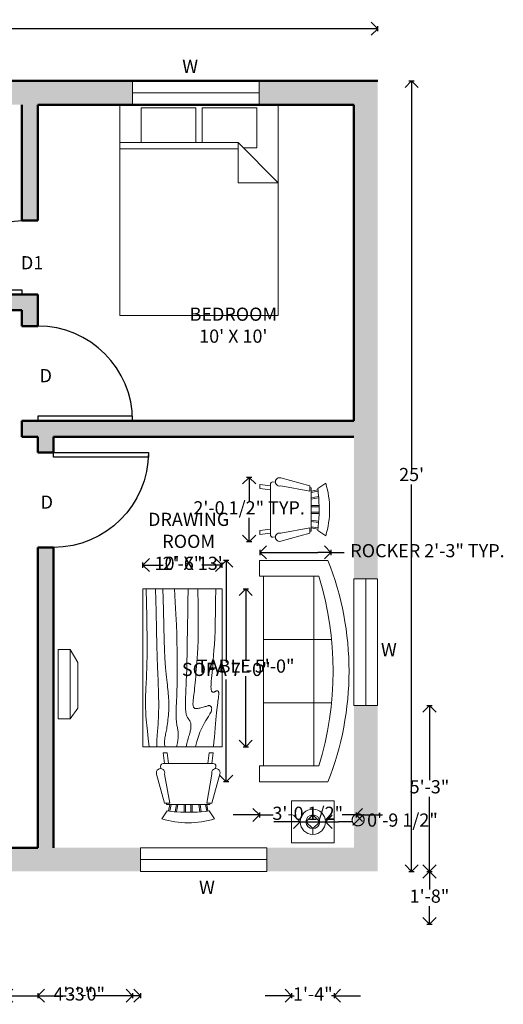
# Model space of a CAD drawing. Units: inches. Extents: x 2691 to 3149, y 584 to 962.
# Tile 3 of 3: x 2966 to 3149, y 588 to 962. Entities that reach past the tile are written whole.
import ezdxf

# ---------------------------------------------------------------- set-up
doc = ezdxf.new("R2010")
doc.units = ezdxf.units.IN
for name, color, linetype, lineweight in [('A-ANNO-DIMS', 2, 'Continuous', 18), ('A-ANNO-TEXT', 159, 'Continuous', 18), ('A-AREA-IDEN', 7, 'Continuous', 25), ('A-DOOR', 4, 'Continuous', 25), ('A-EQPM', 8, 'Continuous', 18), ('A-FURN', 8, 'Continuous', 18), ('A-GLAZ', 40, 'Continuous', 18), ('A-WALL', 254, 'Continuous', 50), ('A-WALL-PATT', 252, 'Continuous', 13)]:
    doc.layers.add(name, color=color, linetype=linetype, lineweight=lineweight)
doc.styles.get("Standard").update_dxf_attribs({"font": 'arial.ttf'})
doc.dimstyles.new('ISO-25', dxfattribs={"dimtxt": 5, "dimasz": 5, "dimexe": 1, "dimexo": 1, "dimtad": 0, "dimtih": 1, "dimtoh": 1, "dimdec": 1, "dimlunit": 3, "dimtxsty": 'Standard', "dimblk": 'OPEN90', "dimcen": 2.5, "dimclrd": 1, "dimclre": 1, "dimclrt": 1, "dimadec": 0, "dimazin": 0, "dimtfac": 1, "dimtdec": 1, "dimtmove": 0, "dimatfit": 3, "dimfxl": 1, "dimfxlon": 1, "dimarcsym": 0})

# ---------------------------------------------------------------- blocks, each defined once
blk = doc.blocks.new('*U5')
for p, q in [((0, 0), (0, -6)), ((-36, 0), (-36, -6))]:
    blk.add_line(p, q)
blk.add_lwpolyline([(0, 0), (0, 36), (-1.75, 36), (-1.75, 0)], close=True)
blk.add_arc((0, 0), 36, 90, 180)
blk = doc.blocks.new('*U4')
for p, q in [((-28, 0), (-28, -6)), ((0, 0), (0, -6))]:
    blk.add_line(p, q)
blk.add_lwpolyline([(0, 0), (0, 28), (-1.75, 28), (-1.75, 0)], close=True)
blk.add_arc((0, 0), 28, 90, 180)
blk = doc.blocks.new('Bed - Queen')
for p, q in [((0, -80.00003), (0, 0)), ((0, 0), (59.99999, 0)), ((59.99999, 0), (59.99999, -80.00003)), ((7.99999, -1.2), (28.79998, -1.2)), ((7.99999, -14.4), (7.99999, -1.2)), ((28.79998, -1.2), (28.79998, -14.4)), ((31.19999, -1.2), (51.99999, -1.2)), ((31.19999, -14.4), (31.19999, -1.2)), ((51.99999, -1.2), (51.99999, -16.4)), ((0, -14.4), (44.8, -14.4)), ((59.99999, -29.6), (44.8, -14.4)), ((44.8, -14.4), (44.8, -29.6)), ((44.8, -16.8), (0, -16.8)), ((51.99999, -16.4), (46.79936, -16.4)), ((44.8, -29.6), (59.99999, -29.6)), ((59.99999, -80.00003), (0, -80.00003))]:
    blk.add_line(p, q)
blk = doc.blocks.new('Sofa - Roundback 7 ft.')
for p, q in [((-12.00002, -32.4421), (-12.00003, -6.5971)), ((11.99997, -32.4421), (11.99998, -6.5971)), ((-36.000027, -34), (-36.000027, -11.4696)), ((-35.999844, -13.3819), (35.9998, -13.3819)), ((35.99998, -34), (35.99998, -11.4696)), ((-36.000027, -32.4421), (35.99998, -32.4421))]:
    blk.add_line(p, q)
for points in [[(-36.000027, -34), (-42.000027, -34), (-42.000027, -8)], [(41.99998, -8), (41.99998, -34), (35.99998, -34)]]:
    blk.add_lwpolyline(points)
for centre, radius, start, end in [((0, -114.25), 114.25, 68.43141, 111.5686), ((-0.00001, -127.1968), 121.1968, 72.72033, 107.2797)]:
    blk.add_arc(centre, radius, start, end)
blk = doc.blocks.new('Table - Rectangular Woodgrain 60 x 30 in.')
for p, q in [((0, 0), (0, -30)), ((60, 0), (0, 0)), ((60, -30), (60, 0)), ((0, -30), (60, -30))]:
    blk.add_line(p, q)
for points in [[(0, -2.4), (4.8155, -2.418), (9.0302, -2.4688), (12.709, -2.5477), (15.9167, -2.65), (18.7181, -2.7711), (21.1781, -2.9063), (23.3616, -3.0508), (25.3333, -3.2), (27.1477, -3.3495), (28.8172, -3.4958), (30.3437, -3.636), (31.7291, -3.7667), (32.9756, -3.8849), (34.0849, -3.9875), (35.059, -4.0714), (35.9, -4.1334), (36.6114, -4.1711), (37.2041, -4.1854), (37.6906, -4.1779), (38.0833, -4.15), (38.3948, -4.1034), (38.6375, -4.0396), (38.8239, -3.9602), (38.9666, -3.8667), (39.0764, -3.7608), (39.1573, -3.6448), (39.2116, -3.521), (39.2416, -3.3917), (39.2498, -3.2593), (39.2385, -3.1261), (39.21, -2.9944), (39.1666, -2.8667), (39.111, -2.7447), (39.0468, -2.6281), (38.978, -2.5163), (38.9083, -2.4083), (38.8418, -2.3035), (38.7823, -2.201), (38.7337, -2.1001), (38.7, -2), (38.6844, -1.9003), (38.6875, -1.8021), (38.7094, -1.707), (38.75, -1.6167), (38.8094, -1.5326), (38.8875, -1.4563), (38.9844, -1.3893), (39.1, -1.3333), (39.2351, -1.2896), (39.3937, -1.2583), (39.5804, -1.2396), (39.8, -1.2333), (40.057, -1.2396), (40.3562, -1.2583), (40.7023, -1.2896), (41.1, -1.3333), (41.5547, -1.3895), (42.0755, -1.4573), (42.6721, -1.5361), (43.3542, -1.625), (44.1316, -1.7233), (45.014, -1.8302), (46.0114, -1.9449), (47.1333, -2.0667), (48.3862, -2.1947), (49.7625, -2.3281), (51.2513, -2.4663), (52.8416, -2.6083), (54.5226, -2.7535), (56.2833, -2.9011), (58.1127, -3.0501), (60, -3.2)], [(0, -9.2), (6.5759, -9.0858), (11.9385, -9.0365), (16.2527, -9.0418), (19.6833, -9.0917), (22.3952, -9.1759), (24.5531, -9.2844), (26.322, -9.4069), (27.8666, -9.5333), (29.3241, -9.6553), (30.7203, -9.7719), (32.0532, -9.8837), (33.3208, -9.9917), (34.5213, -10.0965), (35.6526, -10.199), (36.7128, -10.2999), (37.7, -10.4), (38.6129, -10.4996), (39.4531, -10.5969), (40.223, -10.6895), (40.925, -10.775), (41.5613, -10.8512), (42.1344, -10.9156), (42.6465, -10.966), (43.1, -11), (43.4976, -11.0158), (43.8437, -11.0136), (44.143, -10.9942), (44.4, -10.9583), (44.6195, -10.9069), (44.8062, -10.8406), (44.9648, -10.7603), (45.1, -10.6667), (45.2155, -10.5598), (45.3114, -10.4365), (45.3871, -10.2929), (45.4416, -10.125), (45.4743, -9.929), (45.4844, -9.7011), (45.4709, -9.4371), (45.4333, -9.1333), (45.3716, -8.7883), (45.2896, -8.4104), (45.1919, -8.0107), (45.0833, -7.6), (44.9685, -7.1893), (44.8521, -6.7896), (44.7388, -6.4117), (44.6333, -6.0667), (44.54, -5.7628), (44.4614, -5.4979), (44.4001, -5.2675), (44.3583, -5.0667), (44.3384, -4.8909), (44.3427, -4.7354), (44.3736, -4.5956), (44.4333, -4.4667), (44.5236, -4.3453), (44.6427, -4.2333), (44.7884, -4.1339), (44.9583, -4.05), (45.1501, -3.9849), (45.3614, -3.9417), (45.59, -3.9234), (45.8333, -3.9333), (46.0915, -3.9749), (46.3734, -4.0531), (46.6906, -4.1736), (47.0542, -4.3417), (47.4756, -4.5629), (47.9661, -4.8427), (48.5372, -5.1866), (49.2, -5.6), (49.9676, -6.0844), (50.8594, -6.625), (51.8965, -7.2031), (53.1, -7.8), (54.491, -8.3969), (56.0906, -8.975), (57.9199, -9.5156), (60, -10)], [(0, -12.8), (5.1847, -12.9322), (9.6213, -13.0323), (13.3963, -13.1059), (16.5958, -13.1583), (19.3063, -13.1952), (21.614, -13.2219), (23.6054, -13.2439), (25.3666, -13.2667), (26.9728, -13.2947), (28.4531, -13.3281), (29.8256, -13.3663), (31.1083, -13.4083), (32.3191, -13.4535), (33.476, -13.501), (34.597, -13.5501), (35.7, -13.6), (36.7984, -13.6497), (37.8875, -13.6979), (38.9578, -13.743), (40, -13.7833), (41.0047, -13.8174), (41.9625, -13.8438), (42.864, -13.8607), (43.7, -13.8667), (44.4631, -13.8604), (45.1552, -13.8417), (45.7801, -13.8104), (46.3416, -13.7667), (46.8439, -13.7104), (47.2906, -13.6417), (47.6858, -13.5604), (48.0333, -13.4667), (48.3375, -13.3608), (48.6042, -13.2448), (48.8396, -13.121), (49.05, -12.9917), (49.2417, -12.8593), (49.4208, -12.7261), (49.5937, -12.5944), (49.7667, -12.4667), (49.9452, -12.3451), (50.1323, -12.2313), (50.3303, -12.1268), (50.5416, -12.0333), (50.7686, -11.9524), (51.0135, -11.8854), (51.2788, -11.8341), (51.5666, -11.8), (51.8785, -11.7843), (52.2116, -11.7865), (52.562, -11.8059), (52.926, -11.8417), (53.2998, -11.8931), (53.6795, -11.9594), (54.0614, -12.0397), (54.4416, -12.1333), (54.8223, -12.2401), (55.2293, -12.3625), (55.6942, -12.5037), (56.2489, -12.6667), (56.9251, -12.8547), (57.7545, -13.0708), (58.7689, -13.3182), (60, -13.6)], [(0, -18), (5.124, -17.7273), (9.6609, -17.5057), (13.6705, -17.3303), (17.2125, -17.1958), (20.3467, -17.0973), (23.1328, -17.0297), (25.6307, -16.9878), (27.9, -16.9667), (29.9928, -16.9617), (31.9302, -16.9703), (33.7254, -16.9907), (35.3917, -17.0208), (36.9423, -17.0588), (38.3906, -17.1026), (39.7499, -17.1503), (41.0333, -17.2), (42.2519, -17.2496), (43.4073, -17.2969), (44.4986, -17.3395), (45.525, -17.375), (46.4858, -17.4012), (47.3802, -17.4156), (48.2074, -17.416), (48.9667, -17.4), (49.6583, -17.3662), (50.2872, -17.3167), (50.8595, -17.2547), (51.3812, -17.1833), (51.8584, -17.1057), (52.2971, -17.025), (52.7034, -16.9443), (53.0833, -16.8667), (53.443, -16.7951), (53.789, -16.7313), (54.128, -16.6768), (54.4666, -16.6334), (54.8115, -16.6024), (55.1693, -16.5854), (55.5465, -16.5841), (55.95, -16.6), (56.3828, -16.6337), (56.8346, -16.6823), (57.2915, -16.7418), (57.7396, -16.8084), (58.165, -16.878), (58.5539, -16.9469), (58.8924, -17.0111), (59.1666, -17.0667), (59.3679, -17.1107), (59.5078, -17.1438), (59.6032, -17.1675), (59.6708, -17.1833), (59.7275, -17.193), (59.7901, -17.1979), (59.8753, -17.1998), (60, -17.2)], [(0, -22.4), (8.0098, -22.2501), (14.4094, -22.1011), (19.4168, -21.9535), (23.25, -21.8083), (26.1269, -21.6663), (28.2656, -21.5281), (29.884, -21.3947), (31.2, -21.2667), (32.3967, -21.1448), (33.5172, -21.0292), (34.5697, -20.9198), (35.5625, -20.8167), (36.5037, -20.7198), (37.4015, -20.6292), (38.2642, -20.5448), (39.1, -20.4667), (39.9164, -20.3951), (40.7187, -20.3313), (41.5117, -20.2768), (42.3, -20.2333), (43.0883, -20.2024), (43.8812, -20.1854), (44.6836, -20.1841), (45.5, -20.2), (46.3328, -20.234), (47.1747, -20.2844), (48.0163, -20.3488), (48.8479, -20.425), (49.66, -20.5106), (50.4429, -20.6031), (51.1872, -20.7004), (51.8833, -20.8), (52.5246, -20.8999), (53.1166, -20.9995), (53.6681, -21.0983), (54.1875, -21.1958), (54.6834, -21.2919), (55.1646, -21.3859), (55.6394, -21.4777), (56.1167, -21.5667), (56.6028, -21.6515), (57.0961, -21.7266), (57.5929, -21.7852), (58.0896, -21.8208), (58.5823, -21.8268), (59.0674, -21.7964), (59.5412, -21.723), (60, -21.6)], [(0, -25.2), (8.6355, -25.0504), (15.7026, -24.9031), (21.4049, -24.7606), (25.9458, -24.625), (29.529, -24.4988), (32.3578, -24.3844), (34.6359, -24.284), (36.5667, -24.2), (38.3213, -24.1341), (39.9417, -24.0854), (41.437, -24.0523), (42.8167, -24.0333), (44.0901, -24.0268), (45.2667, -24.0313), (46.3557, -24.0451), (47.3667, -24.0667), (48.309, -24.0947), (49.1928, -24.1287), (50.0284, -24.168), (50.826, -24.2125), (51.5959, -24.2617), (52.3483, -24.3151), (53.0935, -24.3725), (53.8417, -24.4334), (54.6009, -24.497), (55.3699, -24.561), (56.1454, -24.6226), (56.9239, -24.6792), (57.7021, -24.7279), (58.4764, -24.7662), (59.2435, -24.7911), (60, -24.8)], [(0, -28.8), (5.6867, -28.6681), (10.45, -28.5698), (14.407, -28.5012), (17.675, -28.4584), (20.3711, -28.4374), (22.6125, -28.4344), (24.5164, -28.4455), (26.2, -28.4667), (27.762, -28.4947), (29.2276, -28.5281), (30.6033, -28.5663), (31.8958, -28.6084), (33.1118, -28.6535), (34.2578, -28.7011), (35.3405, -28.7501), (36.3666, -28.8), (37.3443, -28.8497), (38.288, -28.8974), (39.2137, -28.9412), (40.1375, -28.9792), (41.0753, -29.0093), (42.0432, -29.0297), (43.0572, -29.0384), (44.1333, -29.0333), (45.2936, -29.0114), (46.5843, -28.9641), (48.0579, -28.8816), (49.7666, -28.7542), (51.7629, -28.5721), (54.0989, -28.3255), (56.8272, -28.0048), (60, -27.6)]]:
    blk.add_lwpolyline(points)
blk = doc.blocks.new('Chair - Rocking')
for p, q in [((-8, -4.5), (-10, -1.5)), ((8, -4.5), (10, -1.5)), ((-8.23428, -6.99939), (-8.3093, -7.47958)), ((-8.23041, -7), (8.23915, -7)), ((-7.5, -4.5), (-7, -7)), ((-6.5, -7), (-7.02225, -4.43)), ((-4.5, -7), (-4.96674, -4.19951)), ((-4, -7), (-4.40532, -4.16272)), ((-1.5, -4.05012), (-1.5, -7)), ((-1, -7), (-1, -4.05012)), ((1, -7), (1, -4.04655)), ((1.5, -4.05012), (1.5, -7)), ((4, -7), (4.40187, -4.18694)), ((4.5, -7), (4.96761, -4.19437)), ((6.5, -7), (7, -4.4057)), ((7.5, -4.5), (7, -7)), ((8.31071, -7.48854), (8.23449, -7.00073)), ((-9, -7.5), (-12, -18.49999)), ((-7, -7.5), (-9, -7.5)), ((-9, -18.49999), (-7, -7.5)), ((7, -7.5), (9, -7.5)), ((9, -18.49999), (7, -7.5)), ((9, -7.5), (12, -18.49999)), ((-10.36644, -20.64523), (-10.5, -21.49999)), ((10.5, -21.49999), (10.3575, -20.58798)), ((-9, -22.49999), (-9.5, -26.49999)), ((0, -22.49999), (-9.5, -22.49999)), ((-8, -26.49999), (-7.5, -22.49999)), ((0, -22.49999), (9.5, -22.49999)), ((8, -26.49999), (7.5, -22.49999)), ((9, -22.49999), (9.5, -26.49999)), ((-9.5, -26.49999), (-8, -26.49999)), ((9.5, -26.49999), (8, -26.49999))]:
    blk.add_line(p, q)
for centre, radius, start, end in [((0, -34.08333), 34.08333, 72.93847, 107.0615), ((0, -68.25004), 64.25, 93.92211, 97.15267), ((0, -68.25004), 64.25, 82.84733, 93.92211), ((-10.5, -18.99999), 1.58114, 161.5651, 18.43495), ((10.5, -18.99999), 1.58114, 161.5651, 18.43495), ((-9.5, -21.49999), 1, 180, 270), ((9.5, -21.49999), 1, 270, 0)]:
    blk.add_arc(centre, radius, start, end)
blk = doc.blocks.new('_Open90')
at = {"color": 0, "linetype": 'ByBlock', "lineweight": -2}
for p, q in [((0, 0), (-1, 0)), ((-0.5, 0.5), (0, 0)), ((0, 0), (-0.5, -0.5))]:
    blk.add_line(p, q, dxfattribs=at)
blk = doc.blocks.new('*D15')
at = {"layer": 'A-ANNO-DIMS', "color": 0, "lineweight": -2, "transparency": 16777216}
for p, q in [((2741.63, 957.65), (2741.63, 959.65)), ((2746.63, 958.65), (2916.78, 958.65)), ((3096.65, 958.65), (2926.51, 958.65)), ((3101.65, 957.65), (3101.65, 959.65))]:
    blk.add_line(p, q, dxfattribs=at)
at = {"layer": 'Defpoints', "color": 0, "transparency": 16777216}
for p in [(2741.63, 958.65), (2741.63, 938.8), (3101.65, 938.8)]:
    blk.add_point(p, dxfattribs=at)
at = {"layer": 'A-ANNO-DIMS', "color": 0, "lineweight": -2, "transparency": 16777216, "xscale": 5, "yscale": 5, "zscale": 5, "rotation": 180}
blk.add_blockref('_Open90', (2741.63, 958.65), dxfattribs=at)
at = {"layer": 'A-ANNO-DIMS', "color": 0, "lineweight": -2, "transparency": 16777216, "xscale": 5, "yscale": 5, "zscale": 5}
blk.add_blockref('_Open90', (3101.65, 958.65), dxfattribs=at)
at = {"layer": 'A-ANNO-DIMS', "color": 0, "transparency": 16777216, "insert": (2921.64, 958.65), "char_height": 5, "attachment_point": 5}
blk.add_mtext("30'", dxfattribs=at)
blk = doc.blocks.new('*D16')
at = {"layer": 'A-ANNO-DIMS', "color": 0, "lineweight": -2, "transparency": 16777216}
for p, q in [((3113.51, 938.8), (3115.51, 938.8)), ((3114.51, 933.8), (3114.51, 791.98)), ((3114.51, 643.8), (3114.51, 785.62)), ((3113.51, 638.8), (3115.51, 638.8))]:
    blk.add_line(p, q, dxfattribs=at)
at = {"layer": 'Defpoints', "color": 0, "transparency": 16777216}
for p in [(3101.65, 938.8), (3101.65, 638.8), (3114.51, 638.8)]:
    blk.add_point(p, dxfattribs=at)
at = {"layer": 'A-ANNO-DIMS', "color": 0, "lineweight": -2, "transparency": 16777216, "xscale": 5, "yscale": 5, "zscale": 5}
for p, rotation in [((3114.51, 938.8), 90), ((3114.51, 638.8), 270)]:
    blk.add_blockref('_Open90', p, dxfattribs=dict(at, rotation=rotation))
at = {"layer": 'A-ANNO-DIMS', "color": 0, "transparency": 16777216, "insert": (3114.51, 788.8), "char_height": 5, "attachment_point": 5}
blk.add_mtext("25'", dxfattribs=at)
blk = doc.blocks.new('WIN-48IN')
for p, q in [((0, 0), (0, 48)), ((0, 48), (9, 48)), ((4.5, 48), (4.5, 0)), ((9, 0), (9, 48)), ((0, 0), (9, 0))]:
    blk.add_line(p, q)
blk = doc.blocks.new('*D26')
at = {"layer": 'A-ANNO-DIMS', "color": 1, "lineweight": -2, "transparency": 16777216}
for p, q in [((3056.9, 760.9), (3056.9, 758.9)), ((3061.9, 759.9), (3078.9, 759.9)), ((3083.9, 760.9), (3083.9, 758.9)), ((3083.9, 759.9), (3088.9, 759.9))]:
    blk.add_line(p, q, dxfattribs=at)
at = {"layer": 'Defpoints', "color": 0, "transparency": 16777216}
for p in [(3056.9, 763.95), (3083.9, 763.95), (3083.9, 759.9)]:
    blk.add_point(p, dxfattribs=at)
at = {"layer": 'A-ANNO-DIMS', "color": 1, "lineweight": -2, "transparency": 16777216, "xscale": 5, "yscale": 5, "zscale": 5, "rotation": 180}
blk.add_blockref('_Open90', (3056.9, 759.9), dxfattribs=at)
at = {"layer": 'A-ANNO-DIMS', "color": 1, "lineweight": -2, "transparency": 16777216, "xscale": 5, "yscale": 5, "zscale": 5}
blk.add_blockref('_Open90', (3083.9, 759.9), dxfattribs=at)
at = {"layer": 'A-ANNO-DIMS', "color": 1, "transparency": 16777216, "insert": (3120.54, 759.9), "char_height": 5, "attachment_point": 5}
blk.add_mtext('ROCKER 2\'-3" TYP.', dxfattribs=at)
blk = doc.blocks.new('*D27')
at = {"layer": 'A-ANNO-DIMS', "color": 1, "lineweight": -2, "transparency": 16777216}
for p, q in [((3053.85, 788.38), (3051.85, 788.38)), ((3052.85, 783.38), (3052.85, 779.37)), ((3052.85, 768.95), (3052.85, 772.95)), ((3053.85, 763.95), (3051.85, 763.95))]:
    blk.add_line(p, q, dxfattribs=at)
at = {"layer": 'Defpoints', "color": 0, "transparency": 16777216}
for p in [(3056.9, 788.38), (3052.85, 763.95), (3056.9, 763.95)]:
    blk.add_point(p, dxfattribs=at)
at = {"layer": 'A-ANNO-DIMS', "color": 1, "lineweight": -2, "transparency": 16777216, "xscale": 5, "yscale": 5, "zscale": 5}
for p, rotation in [((3052.85, 788.38), 90), ((3052.85, 763.95), 270)]:
    blk.add_blockref('_Open90', p, dxfattribs=dict(at, rotation=rotation))
at = {"layer": 'A-ANNO-DIMS', "color": 1, "transparency": 16777216, "insert": (3052.85, 776.16), "char_height": 5, "attachment_point": 5}
blk.add_mtext('2\'-0 1/2" TYP.', dxfattribs=at)
blk = doc.blocks.new('*D32')
at = {"layer": 'A-ANNO-DIMS', "color": 1, "lineweight": -2, "transparency": 16777216}
for p, q in [((3045.16, 756.84), (3043.16, 756.84)), ((3044.16, 751.84), (3044.16, 718.06)), ((3044.16, 677.84), (3044.16, 711.63)), ((3045.16, 672.84), (3043.16, 672.84))]:
    blk.add_line(p, q, dxfattribs=at)
at = {"layer": 'Defpoints', "color": 0, "transparency": 16777216}
for p in [(3056.76, 756.84), (3044.16, 672.84), (3056.76, 672.84)]:
    blk.add_point(p, dxfattribs=at)
at = {"layer": 'A-ANNO-DIMS', "color": 1, "lineweight": -2, "transparency": 16777216, "xscale": 5, "yscale": 5, "zscale": 5}
for p, rotation in [((3044.16, 756.84), 90), ((3044.16, 672.84), 270)]:
    blk.add_blockref('_Open90', p, dxfattribs=dict(at, rotation=rotation))
at = {"layer": 'A-ANNO-DIMS', "color": 1, "transparency": 16777216, "insert": (3044.16, 714.84), "char_height": 5, "attachment_point": 5}
blk.add_mtext('SOFA 7\'-0"', dxfattribs=at)
blk = doc.blocks.new('*D33')
at = {"layer": 'A-ANNO-DIMS', "color": 1, "lineweight": -2, "transparency": 16777216}
for p, q in [((3051.76, 660.24), (3046.76, 660.24)), ((3056.76, 661.24), (3056.76, 659.24)), ((3056.76, 660.24), (3062, 660.24)), ((3093.43, 660.24), (3088.19, 660.24)), ((3093.43, 661.24), (3093.43, 659.24)), ((3098.43, 660.24), (3103.43, 660.24))]:
    blk.add_line(p, q, dxfattribs=at)
at = {"layer": 'Defpoints', "color": 0, "transparency": 16777216}
for p in [(3056.76, 672.84), (3093.43, 672.84), (3093.43, 660.24)]:
    blk.add_point(p, dxfattribs=at)
at = {"layer": 'A-ANNO-DIMS', "color": 1, "lineweight": -2, "transparency": 16777216, "xscale": 5, "yscale": 5, "zscale": 5}
blk.add_blockref('_Open90', (3056.76, 660.24), dxfattribs=at)
at = {"layer": 'A-ANNO-DIMS', "color": 1, "lineweight": -2, "transparency": 16777216, "xscale": 5, "yscale": 5, "zscale": 5, "rotation": 180}
blk.add_blockref('_Open90', (3093.43, 660.24), dxfattribs=at)
at = {"layer": 'A-ANNO-DIMS', "color": 1, "transparency": 16777216, "insert": (3075.1, 660.24), "char_height": 5, "attachment_point": 5}
blk.add_mtext('3\'-0 1/2"', dxfattribs=at)
blk = doc.blocks.new('*D34')
at = {"layer": 'A-ANNO-DIMS', "color": 1, "lineweight": -2, "transparency": 16777216}
for p, q in [((3050.56, 746.1), (3052.56, 746.1)), ((3051.56, 741.1), (3051.56, 719.28)), ((3051.56, 691.1), (3051.56, 712.92)), ((3050.56, 686.1), (3052.56, 686.1))]:
    blk.add_line(p, q, dxfattribs=at)
at = {"layer": 'Defpoints', "color": 0, "transparency": 16777216}
for p in [(3042.56, 746.1), (3042.56, 686.1), (3051.56, 686.1)]:
    blk.add_point(p, dxfattribs=at)
at = {"layer": 'A-ANNO-DIMS', "color": 1, "lineweight": -2, "transparency": 16777216, "xscale": 5, "yscale": 5, "zscale": 5}
for p, rotation in [((3051.56, 746.1), 90), ((3051.56, 686.1), 270)]:
    blk.add_blockref('_Open90', p, dxfattribs=dict(at, rotation=rotation))
at = {"layer": 'A-ANNO-DIMS', "color": 1, "transparency": 16777216, "insert": (3051.56, 716.1), "char_height": 5, "attachment_point": 5}
blk.add_mtext('TABLE 5\'-0"', dxfattribs=at)
blk = doc.blocks.new('*D35')
at = {"layer": 'A-ANNO-DIMS', "color": 1, "lineweight": -2, "transparency": 16777216}
for p, q in [((3012.56, 754.1), (3012.56, 756.1)), ((3017.56, 755.1), (3020.25, 755.1)), ((3037.56, 755.1), (3034.88, 755.1)), ((3042.56, 754.1), (3042.56, 756.1))]:
    blk.add_line(p, q, dxfattribs=at)
at = {"layer": 'Defpoints', "color": 0, "transparency": 16777216}
for p in [(3042.56, 755.1), (3012.56, 746.1), (3042.56, 746.1)]:
    blk.add_point(p, dxfattribs=at)
at = {"layer": 'A-ANNO-DIMS', "color": 1, "lineweight": -2, "transparency": 16777216, "xscale": 5, "yscale": 5, "zscale": 5, "rotation": 180}
blk.add_blockref('_Open90', (3012.56, 755.1), dxfattribs=at)
at = {"layer": 'A-ANNO-DIMS', "color": 1, "lineweight": -2, "transparency": 16777216, "xscale": 5, "yscale": 5, "zscale": 5}
blk.add_blockref('_Open90', (3042.56, 755.1), dxfattribs=at)
at = {"layer": 'A-ANNO-DIMS', "color": 1, "transparency": 16777216, "insert": (3027.56, 755.1), "char_height": 5, "attachment_point": 5}
blk.add_mtext('2\'-6"', dxfattribs=at)
blk = doc.blocks.new('*D47')
at = {"layer": 'A-ANNO-DIMS', "color": 1, "lineweight": -2, "transparency": 16777216}
for p, q in [((3120.3, 701.8), (3122.3, 701.8)), ((3121.3, 696.8), (3121.3, 673.48)), ((3121.3, 643.8), (3121.3, 667.12)), ((3120.3, 638.8), (3122.3, 638.8))]:
    blk.add_line(p, q, dxfattribs=at)
at = {"layer": 'Defpoints', "color": 0, "transparency": 16777216}
for p in [(3101.63, 701.8), (3121.3, 701.8), (3059.63, 638.8)]:
    blk.add_point(p, dxfattribs=at)
at = {"layer": 'A-ANNO-DIMS', "color": 1, "lineweight": -2, "transparency": 16777216, "xscale": 5, "yscale": 5, "zscale": 5}
for p, rotation in [((3121.3, 701.8), 90), ((3121.3, 638.8), 270)]:
    blk.add_blockref('_Open90', p, dxfattribs=dict(at, rotation=rotation))
at = {"layer": 'A-ANNO-DIMS', "color": 1, "transparency": 16777216, "insert": (3121.3, 670.3), "char_height": 5, "attachment_point": 5}
blk.add_mtext('5\'-3"', dxfattribs=at)
blk = doc.blocks.new('*D48')
at = {"layer": 'A-ANNO-DIMS', "color": 1, "lineweight": -2, "transparency": 16777216}
for p, q in [((2960.63, 592.67), (2960.63, 590.67)), ((2965.63, 591.67), (2978.76, 591.67)), ((3006.63, 591.67), (2993.5, 591.67)), ((3011.63, 592.67), (3011.63, 590.67))]:
    blk.add_line(p, q, dxfattribs=at)
at = {"layer": 'Defpoints', "color": 0, "transparency": 16777216}
for p in [(2960.63, 638.8), (3011.63, 638.8), (3011.63, 591.67)]:
    blk.add_point(p, dxfattribs=at)
at = {"layer": 'A-ANNO-DIMS', "color": 1, "lineweight": -2, "transparency": 16777216, "xscale": 5, "yscale": 5, "zscale": 5, "rotation": 180}
blk.add_blockref('_Open90', (2960.63, 591.67), dxfattribs=at)
at = {"layer": 'A-ANNO-DIMS', "color": 1, "lineweight": -2, "transparency": 16777216, "xscale": 5, "yscale": 5, "zscale": 5}
blk.add_blockref('_Open90', (3011.63, 591.67), dxfattribs=at)
at = {"layer": 'A-ANNO-DIMS', "color": 1, "transparency": 16777216, "insert": (2986.13, 591.67), "char_height": 5, "attachment_point": 5}
blk.add_mtext('4\'-3"', dxfattribs=at)
blk = doc.blocks.new('*D52')
at = {"layer": 'A-ANNO-DIMS', "color": 1, "lineweight": -2, "transparency": 16777216}
for p, q in [((2972.63, 592.67), (2972.63, 590.67)), ((2977.63, 591.67), (2983.36, 591.67)), ((3003.63, 591.67), (2997.9, 591.67)), ((3008.63, 592.67), (3008.63, 590.67))]:
    blk.add_line(p, q, dxfattribs=at)
at = {"layer": 'Defpoints', "color": 0, "transparency": 16777216}
for p in [(2972.63, 809.8), (3008.63, 809.8), (3008.63, 591.67)]:
    blk.add_point(p, dxfattribs=at)
at = {"layer": 'A-ANNO-DIMS', "color": 1, "lineweight": -2, "transparency": 16777216, "xscale": 5, "yscale": 5, "zscale": 5, "rotation": 180}
blk.add_blockref('_Open90', (2972.63, 591.67), dxfattribs=at)
at = {"layer": 'A-ANNO-DIMS', "color": 1, "lineweight": -2, "transparency": 16777216, "xscale": 5, "yscale": 5, "zscale": 5}
blk.add_blockref('_Open90', (3008.63, 591.67), dxfattribs=at)
at = {"layer": 'A-ANNO-DIMS', "color": 1, "transparency": 16777216, "insert": (2990.63, 591.67), "char_height": 5, "attachment_point": 5}
blk.add_mtext('3\'-0"', dxfattribs=at)
blk = doc.blocks.new('*D55')
at = {"layer": 'A-ANNO-DIMS', "color": 1, "lineweight": -2, "transparency": 16777216}
for p, q in [((3120.3, 638.8), (3122.3, 638.8)), ((3121.3, 633.8), (3121.3, 631.98)), ((3121.3, 623.8), (3121.3, 625.62)), ((3120.3, 618.8), (3122.3, 618.8))]:
    blk.add_line(p, q, dxfattribs=at)
at = {"layer": 'Defpoints', "color": 0, "transparency": 16777216}
for p in [(2964.26, 638.8), (3121.3, 638.8), (2964.26, 618.8)]:
    blk.add_point(p, dxfattribs=at)
at = {"layer": 'A-ANNO-DIMS', "color": 1, "lineweight": -2, "transparency": 16777216, "xscale": 5, "yscale": 5, "zscale": 5}
for p, rotation in [((3121.3, 638.8), 90), ((3121.3, 618.8), 270)]:
    blk.add_blockref('_Open90', p, dxfattribs=dict(at, rotation=rotation))
at = {"layer": 'A-ANNO-DIMS', "color": 1, "transparency": 16777216, "insert": (3121.3, 628.8), "char_height": 5, "attachment_point": 5}
blk.add_mtext('1\'-8"', dxfattribs=at)
blk = doc.blocks.new('*D58')
at = {"layer": 'A-ANNO-DIMS', "color": 1, "lineweight": -2, "transparency": 16777216}
for p, q in [((3063.99, 591.67), (3058.99, 591.67)), ((3068.99, 592.67), (3068.99, 590.67)), ((3068.99, 591.67), (3069.99, 591.67)), ((3085.07, 591.67), (3084.06, 591.67)), ((3085.07, 592.67), (3085.07, 590.67)), ((3090.07, 591.67), (3095.07, 591.67))]:
    blk.add_line(p, q, dxfattribs=at)
at = {"layer": 'Defpoints', "color": 0, "transparency": 16777216}
for p in [(3068.99, 649.7), (3085.07, 649.7), (3085.07, 591.67)]:
    blk.add_point(p, dxfattribs=at)
at = {"layer": 'A-ANNO-DIMS', "color": 1, "lineweight": -2, "transparency": 16777216, "xscale": 5, "yscale": 5, "zscale": 5}
blk.add_blockref('_Open90', (3068.99, 591.67), dxfattribs=at)
at = {"layer": 'A-ANNO-DIMS', "color": 1, "lineweight": -2, "transparency": 16777216, "xscale": 5, "yscale": 5, "zscale": 5, "rotation": 180}
blk.add_blockref('_Open90', (3085.07, 591.67), dxfattribs=at)
at = {"layer": 'A-ANNO-DIMS', "color": 1, "transparency": 16777216, "insert": (3077.03, 591.67), "char_height": 5, "attachment_point": 5}
blk.add_mtext('1\'-4"', dxfattribs=at)
blk = doc.blocks.new('*D59')
at = {"layer": 'A-ANNO-DIMS', "color": 1, "lineweight": -2, "transparency": 16777216}
for p, q in [((3067.23, 657.66), (3062.23, 657.66)), ((3072.23, 657.66), (3081.82, 657.66)), ((3091.82, 657.66), (3086.82, 657.66))]:
    blk.add_line(p, q, dxfattribs=at)
at = {"layer": 'Defpoints', "color": 0, "transparency": 16777216}
for p in [(3072.23, 657.66), (3081.82, 657.66)]:
    blk.add_point(p, dxfattribs=at)
at = {"layer": 'A-ANNO-DIMS', "color": 1, "lineweight": -2, "transparency": 16777216, "xscale": 5, "yscale": 5, "zscale": 5}
for p, rotation in [((3072.23, 657.66), 359.9991277919116), ((3081.82, 657.66), 179.9991277919116)]:
    blk.add_blockref('_Open90', p, dxfattribs=dict(at, rotation=rotation))
at = {"layer": 'A-ANNO-DIMS', "color": 1, "transparency": 16777216, "insert": (3107.64, 657.66), "char_height": 5, "attachment_point": 5}
blk.add_mtext('∅0\'-9 1/2"', dxfattribs=at)

msp = doc.modelspace()

# ---------------------------------------------------------------- hatches: boundary and pattern name
at = {"layer": 'A-WALL-PATT'}
h = msp.add_hatch(color=256, dxfattribs=at)
h.dxf.hatch_style = 1
h.paths.add_polyline_path([(2786.63, 938.8), (2741.63, 938.8), (2741.63, 803.8), (2822.63, 803.8), (2822.63, 785.8), (2828.63, 785.8), (2828.63, 803.8), (2876.63, 803.8), (2876.63, 809.8), (2870.63, 809.8), (2834.63, 809.8), (2750.63, 809.8), (2750.63, 929.8), (2786.63, 929.8)])
h.paths.add_polyline_path([(2885.63, 938.8), (2834.63, 938.8), (2834.63, 929.8), (2840.63, 929.8), (2870.63, 929.8), (2870.63, 885.8), (2876.63, 885.8), (2876.63, 929.8), (2885.63, 929.8)])
h.paths.add_polyline_path([(2933.63, 938.8), (2909.63, 938.8), (2909.63, 929.8), (2918.63, 929.8), (2918.63, 908.89), (2918.64, 908.89), (2918.63, 925.2), (2912.41, 925.19), (2912.43, 908.88), (2918.63, 908.89), (2918.63, 925.2), (2918.63, 925.2), (2918.64, 908.89), (2918.63, 857.8), (2870.63, 857.8), (2870.63, 845.8), (2876.63, 845.8), (2876.63, 851.8), (2966.63, 851.8), (2966.63, 845.8), (2972.63, 845.8), (2972.63, 857.8), (2924.63, 857.8), (2924.63, 929.8), (2933.63, 929.8)])
h.paths.add_polyline_path([(2917.85, 923.84), (2917.86, 910.44, -0.414214), (2917.28, 909.66), (2913.98, 909.66, -0.414214), (2913.2, 910.24), (2913.19, 923.64, -0.414214), (2913.77, 924.42), (2917.07, 924.42, -0.414214)], flags=16)
h.paths.add_polyline_path([(3008.63, 938.8), (2957.63, 938.8), (2957.63, 929.8), (2966.63, 929.8), (2966.63, 885.8), (2972.63, 885.8), (2972.63, 929.8), (3008.63, 929.8)])
h.paths.add_polyline_path([(3101.63, 938.8), (3056.63, 938.8), (3056.63, 929.8), (3063.83, 929.8), (3092.63, 929.8), (3092.63, 809.8), (2966.63, 809.8), (2966.63, 803.8), (2972.63, 803.8), (2972.63, 797.8), (2978.63, 797.8), (2978.63, 803.8), (3092.63, 803.8), (3092.63, 749.8), (3101.63, 749.8)])
h.paths.add_polyline_path([(2828.63, 757.8), (2822.63, 757.8), (2822.63, 755.8), (2741.63, 755.8), (2741.63, 715.3), (2750.63, 715.3), (2750.63, 749.8), (2828.63, 749.8)])
h.paths.add_polyline_path([(2870.63, 734.8), (2864.63, 734.8), (2864.63, 647.8), (2750.63, 647.8), (2750.63, 679.3), (2741.63, 679.3), (2741.63, 638.8), (2870.63, 638.8)])
h.paths.add_polyline_path([(2924.63, 680.8), (2924.63, 734.8), (2918.63, 734.8), (2918.63, 638.8), (2924.63, 638.8), (2924.63, 644.8)])
h.paths.add_polyline_path([(3011.63, 647.8), (2978.63, 647.8), (2978.63, 761.8), (2972.63, 761.8), (2972.63, 647.8), (2960.51, 647.8, -0.020861), (2960.63, 644.8), (2960.63, 638.8), (3011.63, 638.8)])
h.paths.add_polyline_path([(3101.63, 701.8), (3092.63, 701.8), (3092.63, 647.8), (3059.63, 647.8), (3059.63, 638.8), (3101.63, 638.8)])

# ---------------------------------------------------------------- linework, layer by layer
at = {"layer": 'A-EQPM'}
for p, q in [((2984.96, 723.06), (2987.81, 718.13)), ((2987.81, 718.13), (2987.81, 700.81)), ((2987.81, 700.81), (2984.96, 696.78))]:
    msp.add_line(p, q, dxfattribs=at)
msp.add_lwpolyline([(2980.43, 723.06), (2984.96, 723.06), (2984.96, 696.78), (2980.43, 696.78)], close=True, dxfattribs=at)
at = {"layer": 'A-FURN'}
for p, q in [((3077.03, 662.45), (3077.03, 660.26)), ((3072.23, 657.66), (3074.42, 657.66)), ((3074.42, 657.66), (3077.03, 660.26)), ((3077.03, 655.05), (3074.42, 657.66)), ((3077.03, 660.26), (3079.63, 657.66)), ((3079.63, 657.66), (3077.03, 655.05)), ((3079.63, 657.66), (3081.82, 657.66)), ((3077.03, 655.05), (3077.03, 652.86))]:
    msp.add_line(p, q, dxfattribs=at)
msp.add_lwpolyline([(3068.99, 665.62), (3085.07, 665.62), (3085.07, 649.7), (3068.99, 649.7)], close=True, dxfattribs=at)
for radius in [4.8, 2.6]:
    msp.add_circle((3077.03, 657.66), radius, dxfattribs=at)
at = {"layer": 'A-GLAZ'}
for p, q in [((3008.63, 929.8), (3008.63, 938.8)), ((3056.63, 929.8), (3056.63, 938.8)), ((3008.63, 934.3), (3056.63, 934.3))]:
    msp.add_line(p, q, dxfattribs=at)
at = {"layer": 'A-WALL'}
for p, q in [((3056.63, 938.8), (2834.63, 938.8)), ((3056.63, 938.8), (3101.65, 938.8)), ((2966.63, 929.8), (2966.63, 885.8)), ((3092.63, 929.8), (2972.63, 929.8)), ((2972.63, 929.8), (2972.63, 885.8)), ((3092.63, 809.8), (3092.63, 929.8)), ((2966.63, 885.8), (2972.63, 885.8)), ((2972.63, 857.8), (2924.63, 857.8)), ((2972.63, 845.8), (2972.63, 857.8)), ((2966.63, 851.8), (2876.63, 851.8)), ((2966.63, 845.8), (2966.63, 851.8)), ((2966.63, 845.8), (2972.63, 845.8)), ((3092.63, 809.8), (2966.63, 809.8)), ((2966.63, 803.8), (2966.63, 809.8)), ((2972.63, 803.8), (2966.63, 803.8)), ((2972.63, 803.8), (2972.63, 797.8)), ((3092.63, 803.8), (2978.63, 803.8)), ((2978.63, 797.8), (2978.63, 803.8)), ((2972.63, 797.8), (2978.63, 797.8)), ((2972.63, 761.8), (2972.63, 647.8)), ((2972.63, 761.8), (2978.63, 761.8)), ((2978.63, 761.8), (2978.63, 647.8)), ((2960.51, 647.8), (2972.63, 647.8))]:
    msp.add_line(p, q, dxfattribs=at)

# ---------------------------------------------------------------- block references
at = {"layer": 'A-DOOR', "xscale": -1}
for name, p, rotation in [('*U4', (2966.63, 857.8), 90), ('*U5', (2978.63, 797.8), 270)]:
    msp.add_blockref(name, p, dxfattribs=dict(at, rotation=rotation))
at = {"layer": 'A-DOOR', "rotation": 270}
msp.add_blockref('*U5', (2972.63, 809.8), dxfattribs=at)
at = {"layer": 'A-FURN'}
msp.add_blockref('Bed - Queen', (3003.83, 929.8), dxfattribs=at)
at = {"layer": 'A-FURN', "rotation": 270}
for name, p in [('Chair - Rocking', (3083.4, 776.16)), ('Sofa - Roundback 7 ft.', (3090.76, 714.84)), ('Table - Rectangular Woodgrain 60 x 30 in.', (3042.56, 746.1))]:
    msp.add_blockref(name, p, dxfattribs=at)
at = {"layer": 'A-FURN', "xscale": -1, "rotation": 180}
msp.add_blockref('Chair - Rocking', (3029.74, 657.28), dxfattribs=at)
at = {"layer": 'A-GLAZ'}
msp.add_blockref('WIN-48IN', (3092.63, 701.8), dxfattribs=at)
at = {"layer": 'A-GLAZ', "rotation": 270.0000000000025}
msp.add_blockref('WIN-48IN', (3011.63, 647.8), dxfattribs=at)

# ---------------------------------------------------------------- texts
at = {"layer": 'A-ANNO-TEXT', "char_height": 5, "attachment_point": 1}
for s, insert in [('\\pxqc;{W}', (3024.86, 946.87)), ('\\pxqc;{D1}', (2964.89, 872.32)), ('\\pxqc;{D}', (2970.08, 829.47)), ('\\pxqc;{D}', (2970.48, 781.48)), ('\\pxqc;{W}', (3100.27, 725.47)), ('\\pxqc;{W}', (3031.23, 635.29))]:
    msp.add_mtext_dynamic_manual_height_columns(s, width=11.2162, gutter_width=12.5, heights=[0], dxfattribs=dict(at, insert=insert))
at = {"layer": 'A-AREA-IDEN', "char_height": 5, "attachment_point": 1}
for s, width, insert in [("\\pxqc;BEDROOM\\P10' X 10'", 50.6943, (3021.51, 852.8)), ("\\pxqc;DRAWING\\PROOM\\P10' X 13'", 46.9438, (3006.44, 774.93))]:
    msp.add_mtext_dynamic_manual_height_columns(s, width=width, gutter_width=12.5, heights=[0], dxfattribs=dict(at, insert=insert))

# ---------------------------------------------------------------- dimensions: what is measured, and where the dimension line sits
at = {"layer": 'A-ANNO-DIMS'}
for base, p1, p2, override, picture, middle in [((2741.63, 958.65), (3101.65, 938.8), (2741.63, 938.8), {"dimclrd": 0, "dimclre": 0, "dimclrt": 0}, '*D15', (2921.64, 958.65)), ((3008.63, 591.67), (2972.63, 809.8), (3008.63, 809.8), {"dimdec": 1, "dimlfac": 1, "dimrnd": 0, "dimzin": 1, "dimdsep": 46, "dimlunit": 4, "dimfrac": 2}, '*D52', (2990.63, 591.67)), ((3042.56, 755.1), (3012.56, 746.1), (3042.56, 746.1), {"dimdec": 1, "dimlfac": 1, "dimrnd": 0, "dimzin": 1, "dimdsep": 46, "dimlunit": 4, "dimfrac": 2}, '*D35', (3027.56, 755.1)), ((3093.43, 660.24), (3056.76, 672.84), (3093.43, 672.84), {"dimdec": 1, "dimlfac": 1, "dimrnd": 0, "dimzin": 1, "dimdsep": 46, "dimlunit": 4, "dimfrac": 2}, '*D33', (3075.1, 660.24)), ((3085.07, 591.67), (3068.99, 649.7), (3085.07, 649.7), {"dimdec": 1, "dimlfac": 1, "dimrnd": 0, "dimzin": 1, "dimdsep": 46, "dimlunit": 4, "dimfrac": 2}, '*D58', (3077.03, 591.67)), ((3011.63, 591.67), (2960.63, 638.8), (3011.63, 638.8), {"dimdec": 1, "dimlfac": 1, "dimrnd": 0, "dimzin": 1, "dimdsep": 46, "dimlunit": 4, "dimfrac": 2}, '*D48', (2986.13, 591.67))]:
    dim = msp.add_linear_dim(base=base, p1=p1, p2=p2, dimstyle='ISO-25', override=override, dxfattribs=at)
    dim.commit()
    dim.dimension.update_dxf_attribs({"geometry": picture, "text_midpoint": middle})
for base, p1, p2, override, picture, middle in [((3114.51, 638.8), (3101.65, 938.8), (3101.65, 638.8), {"dimclrd": 0, "dimclre": 0, "dimclrt": 0}, '*D16', (3114.51, 788.8)), ((3121.3, 701.8), (3059.63, 638.8), (3101.63, 701.8), {"dimdec": 1, "dimlfac": 1, "dimrnd": 0, "dimzin": 1, "dimdsep": 46, "dimlunit": 4, "dimfrac": 2}, '*D47', (3121.3, 670.3)), ((3121.3, 638.8), (2964.26, 618.8), (2964.26, 638.8), {"dimdec": 1, "dimlfac": 1, "dimrnd": 0, "dimzin": 1, "dimdsep": 46, "dimlunit": 4, "dimfrac": 2}, '*D55', (3121.3, 628.8))]:
    dim = msp.add_linear_dim(base=base, p1=p1, p2=p2, angle=90, dimstyle='ISO-25', override=override, dxfattribs=at)
    dim.commit()
    dim.dimension.update_dxf_attribs({"geometry": picture, "text_midpoint": middle})
for base, p1, p2, text, picture, middle in [((3052.85, 763.95), (3056.9, 788.38), (3056.9, 763.95), '<> TYP.', '*D27', (3052.85, 776.16)), ((3044.16, 672.84), (3056.76, 756.84), (3056.76, 672.84), 'SOFA <>', '*D32', (3044.16, 714.84)), ((3051.56, 686.1), (3042.56, 746.1), (3042.56, 686.1), 'TABLE <>', '*D34', (3051.56, 716.1))]:
    dim = msp.add_linear_dim(base=base, p1=p1, p2=p2, angle=270, text=text, dimstyle='ISO-25', override={"dimdec": 1, "dimlfac": 1, "dimrnd": 0, "dimzin": 1, "dimdsep": 46, "dimlunit": 4, "dimfrac": 2}, dxfattribs=at)
    dim.commit()
    dim.dimension.update_dxf_attribs({"geometry": picture, "text_midpoint": middle})
dim = msp.add_linear_dim(base=(3083.9, 759.9), p1=(3056.9, 763.95), p2=(3083.9, 763.95), text='ROCKER <> TYP.', dimstyle='ISO-25', override={"dimdec": 1, "dimlfac": 1, "dimrnd": 0, "dimzin": 1, "dimdsep": 46, "dimlunit": 4, "dimfrac": 2}, dxfattribs=at)
dim.commit()
dim.dimension.update_dxf_attribs({"geometry": '*D26', "text_midpoint": (3120.54, 759.9)})
dim = msp.add_diameter_dim_2p(p1=(3072.23, 657.66), p2=(3081.82, 657.66), dimstyle='ISO-25', override={"dimdec": 1, "dimlfac": 1, "dimrnd": 0, "dimzin": 1, "dimdsep": 46, "dimlunit": 4, "dimfrac": 2}, dxfattribs=at)
dim.commit()
dim.dimension.update_dxf_attribs({"geometry": '*D59', "text_midpoint": (3091.82, 657.66), "dimtype": 163})

doc.saveas('drawing.dxf')
